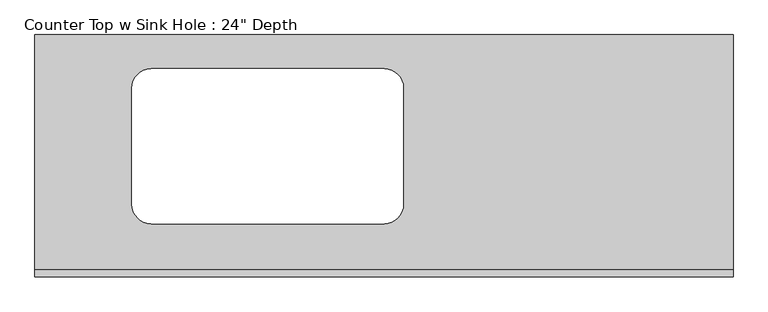
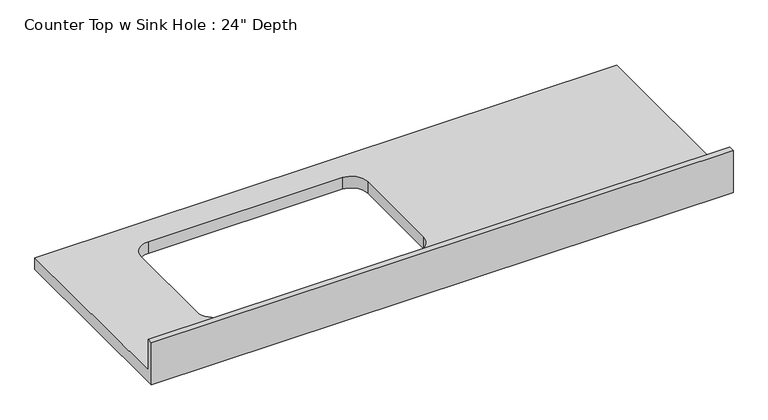
"""IFC4 building model written with IfcOpenShell, lengths in millimetres: furniture geometry."""

from ifc_helpers import new_model, si_unit, frame, origin, place, context, project, spatial, polyline, circle_curve, source, transform, mapped, element, save
from ifc_brep_helpers import plane_surface, revolved_surface, advanced_brep


def furniture_d860a6bd(model_context):
    return source(origin(), model_context, "Body", "AdvancedBrep", [
        advanced_brep(
        [(-1200.4622951, 635.0, 914.4), (-1200.4622951, 19.05, 914.4), (628.3377049, 19.05, 914.4), (628.3377049, 635.0, 914.4), (-895.6622951, 139.7, 914.4), (-946.4622951, 190.5, 914.4), (-946.4622951, 495.3, 914.4), (-895.6622951, 546.1, 914.4), (-286.0622951, 546.1, 914.4), (-235.2622951, 495.3, 914.4), (-235.2622951, 190.5, 914.4), (-286.0622951, 139.7, 914.4), (628.3377049, 0.0, 876.3), (-1200.4622951, 0.0, 876.3), (-1200.4622951, 635.0, 876.3), (628.3377049, 635.0, 876.3), (-286.0622951, 139.7, 876.3), (-235.2622951, 190.5, 876.3), (-235.2622951, 495.3, 876.3), (-286.0622951, 546.1, 876.3), (-895.6622951, 546.1, 876.3), (-946.4622951, 495.3, 876.3), (-946.4622951, 190.5, 876.3), (-895.6622951, 139.7, 876.3), (628.3377049, 0.0, 1016.0), (-1200.4622951, 0.0, 1016.0), (-1200.4622951, 19.05, 1016.0), (628.3377049, 19.05, 1016.0)],
        [
            (0, 1),
            (1, 2),
            (2, 3),
            (3, 0),
            (4, 5, circle_curve(frame((-895.6622951, 190.5, 914.4), z_axis=(0.0, 0.0, -1.0), x_axis=(1.0, 0.0, 0.0)), 50.8)),
            (5, 6),
            (6, 7, circle_curve(frame((-895.6622951, 495.3, 914.4), z_axis=(0.0, 0.0, -1.0), x_axis=(1.0, 0.0, 0.0)), 50.8)),
            (7, 8),
            (8, 9, circle_curve(frame((-286.0622951, 495.3, 914.4), z_axis=(0.0, 0.0, -1.0), x_axis=(1.0, 0.0, 0.0)), 50.8)),
            (9, 10),
            (10, 11, circle_curve(frame((-286.0622951, 190.5, 914.4), z_axis=(0.0, 0.0, -1.0), x_axis=(1.0, 0.0, 0.0)), 50.8)),
            (11, 4),
            (12, 13),
            (13, 14),
            (14, 15),
            (15, 12),
            (16, 17, circle_curve(frame((-286.0622951, 190.5, 876.3), z_axis=(0.0, 0.0, 1.0), x_axis=(1.0, 0.0, 0.0)), 50.8)),
            (17, 18),
            (18, 19, circle_curve(frame((-286.0622951, 495.3, 876.3), z_axis=(0.0, 0.0, 1.0), x_axis=(1.0, 0.0, 0.0)), 50.8)),
            (19, 20),
            (20, 21, circle_curve(frame((-895.6622951, 495.3, 876.3), z_axis=(0.0, 0.0, 1.0), x_axis=(1.0, 0.0, 0.0)), 50.8)),
            (21, 22),
            (22, 23, circle_curve(frame((-895.6622951, 190.5, 876.3), z_axis=(0.0, 0.0, 1.0), x_axis=(1.0, 0.0, 0.0)), 50.8)),
            (23, 16),
            (12, 24),
            (24, 25),
            (25, 13),
            (25, 26),
            (26, 1),
            (0, 14),
            (3, 15),
            (2, 27),
            (27, 24),
            (11, 16),
            (23, 4),
            (22, 5),
            (21, 6),
            (20, 7),
            (19, 8),
            (18, 9),
            (17, 10),
            (27, 26),
        ],
        [
            plane_surface(frame((-1200.4622951, 0.0, 914.4), z_axis=(0.0, 0.0, 1.0), x_axis=(-1.0, 0.0, 0.0))),
            plane_surface(frame((-1200.4622951, 0.0, 876.3), z_axis=(0.0, 0.0, -1.0), x_axis=(1.0, 0.0, 0.0))),
            plane_surface(frame((628.3377049, 0.0, 914.4), z_axis=(0.0, -1.0, 0.0), x_axis=(0.0, 0.0, -1.0))),
            plane_surface(frame((-1200.4622951, 0.0, 914.4), z_axis=(-1.0, 0.0, 0.0), x_axis=(0.0, 0.0, -1.0))),
            plane_surface(frame((-1200.4622951, 635.0, 914.4), z_axis=(0.0, 1.0, 0.0), x_axis=(0.0, 0.0, -1.0))),
            plane_surface(frame((628.3377049, 635.0, 914.4), z_axis=(1.0, 0.0, 0.0), x_axis=(0.0, 0.0, -1.0))),
            plane_surface(frame((-286.0622951, 139.7, 914.4), z_axis=(0.0, 1.0, 0.0), x_axis=(0.0, 0.0, -1.0))),
            revolved_surface(polyline([(-844.8622951000001, 190.5, 914.4), (-844.8622951000001, 190.5, 876.3)]), (-895.6622951, 190.5, 876.3), (0.0, 0.0, 1.0)),
            plane_surface(frame((-946.4622951, 190.5, 914.4), z_axis=(1.0, 0.0, 0.0), x_axis=(0.0, 0.0, -1.0))),
            revolved_surface(polyline([(-844.8622951000001, 495.3, 914.4), (-844.8622951000001, 495.3, 876.3)]), (-895.6622951, 495.3, 876.3), (0.0, 0.0, 1.0)),
            plane_surface(frame((-895.6622951, 546.1, 914.4), z_axis=(0.0, -1.0, 0.0), x_axis=(0.0, 0.0, -1.0))),
            revolved_surface(polyline([(-235.26229509999996, 495.3, 914.4), (-235.26229509999996, 495.3, 876.3)]), (-286.0622951, 495.3, 876.3), (0.0, 0.0, 1.0)),
            plane_surface(frame((-235.2622951, 495.3, 914.4), z_axis=(-1.0, 0.0, 0.0), x_axis=(0.0, 0.0, -1.0))),
            revolved_surface(polyline([(-235.26229509999996, 190.5, 914.4), (-235.26229509999996, 190.5, 876.3)]), (-286.0622951, 190.5, 876.3), (0.0, 0.0, 1.0)),
            plane_surface(frame((-1200.4622951, 0.0, 1016.0), z_axis=(0.0, 0.0, 1.0), x_axis=(0.0, 1.0, 0.0))),
            plane_surface(frame((-1200.4622951, 19.05, 1016.0), z_axis=(0.0, 1.0, 0.0), x_axis=(0.0, 0.0, -1.0))),
        ],
        [
            (0, [[1, 2, 3, 4], [5, 6, 7, 8, 9, 10, 11, 12]]),
            (1, [[13, 14, 15, 16], [17, 18, 19, 20, 21, 22, 23, 24]]),
            (2, [[25, 26, 27, -13]]),
            (3, [[-27, 28, 29, -1, 30, -14]]),
            (4, [[31, -15, -30, -4]]),
            (5, [[-31, -3, 32, 33, -25, -16]]),
            (6, [[-12, 34, -24, 35]]),
            (7, [[-23, 36, -5, -35]]),
            (8, [[-22, 37, -6, -36]]),
            (9, [[-21, 38, -7, -37]]),
            (10, [[-20, 39, -8, -38]]),
            (11, [[-19, 40, -9, -39]]),
            (12, [[-18, 41, -10, -40]]),
            (13, [[-11, -41, -17, -34]]),
            (14, [[-26, -33, 42, -28]]),
            (15, [[-32, -2, -29, -42]]),
        ],
    ),
    ])


if __name__ == "__main__":
    model = new_model("IFC4")
    model_context = context("Model", 3, world=origin())
    ifc_project = project(units=[si_unit("LENGTHUNIT", "METRE", prefix="MILLI")], contexts=[model_context])
    site = spatial("IfcSite", under=ifc_project)
    building = spatial("IfcBuilding", under=site)
    placement = place(None, origin())
    furniture_shape = furniture_d860a6bd(model_context)
    element("IfcFurniture", 1, ObjectType="Counter Top w Sink Hole : 24\" Depth", at=placement, inside=building, context=model_context, shape_type="MappedRepresentation", body=[
        mapped(furniture_shape, transform((0.0, 0.0, 0.0), x_axis=(1.0, 0.0, 0.0), y_axis=(0.0, 1.0, 0.0), z_axis=(0.0, 0.0, 1.0))),
    ])
    save(model, "model.ifc")

# Revit data of these elements
# Type "Counter Top w Sink Hole : 24\" Depth"
#   Assembly Code = "C1030400"
#   Counter Thickness = 0' - 1 1/2"
#   Depth = 2' - 1"
#   Height = 3' - 0"
#   Length [instance default] = 8' - 0"
#   Sink Location [instance default] = 2' - 0"
#   Sink Location To Wall [instance default] = 0' - 6"
#   Sink Opening Depth [instance default] = 1' - 3"
#   Sink Opening Width [instance default] = 2' - 3"
#   Counter Top Material = none
#   Default Elevation = 0
# Element 1 (IfcFurniture, "Counter Top w Sink Hole : 24\" Depth")
#   Length = 6' - 0"
#   Materials on its faces: "Counter Top"
# Materials
#   "Counter Top": class "Wood", colour RGB 226 177 128, transparency 0
